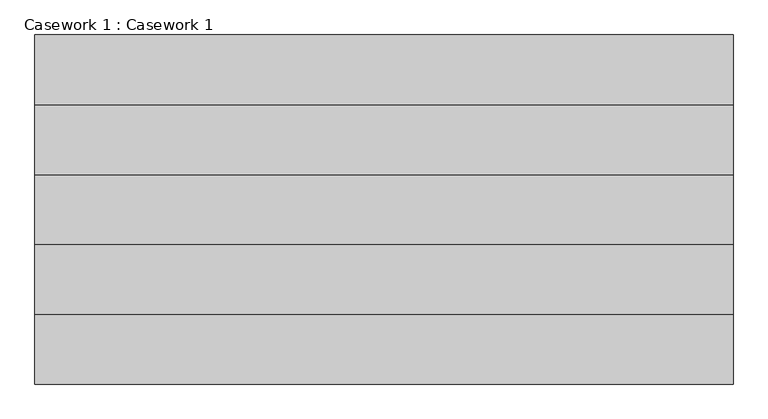
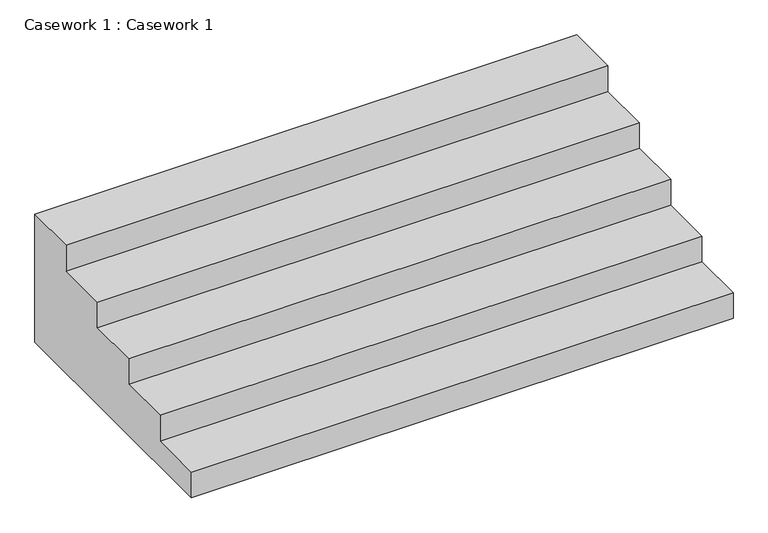
"""IFC4 building model written with IfcOpenShell, lengths in millimetres: furniture geometry, Casework 1 : Casework 1."""

from ifc_helpers import new_model, si_unit, frame, origin, place, context, project, spatial, polyline, outline, extrude, source, transform, mapped, element, save


def casework_1_casework_1_0b0e07b3(model_context):
    return source(origin(), model_context, "Body", "SweptSolid", [
        extrude(outline(polyline([(241.4737487, 2311.4), (546.2737487, 2311.4), (546.2737487, 1549.4), (-977.7262513, 1549.4), (-977.7262513, 1701.8), (-672.9262513, 1701.8), (-672.9262513, 1854.2), (-368.1262513, 1854.2), (-368.1262513, 2006.6), (-63.3262513, 2006.6), (-63.3262513, 2159.0), (241.4737487, 2159.0), (241.4737487, 2311.4)])), frame((-15445.0994093, 0.0, 0.0), z_axis=(1.0, 0.0, 0.0), x_axis=(0.0, 1.0, 0.0)), (0.0, 0.0, 1.0), 3048.0),
    ])


if __name__ == "__main__":
    model = new_model("IFC4")
    model_context = context("Model", 3, world=origin())
    ifc_project = project(units=[si_unit("LENGTHUNIT", "METRE", prefix="MILLI")], contexts=[model_context])
    site = spatial("IfcSite", under=ifc_project)
    building = spatial("IfcBuilding", under=site)
    placement = place(None, origin())
    casework_1_casework_1_shape = casework_1_casework_1_0b0e07b3(model_context)
    element("IfcFurniture", 1, ObjectType="Casework 1 : Casework 1", at=placement, inside=building, context=model_context, shape_type="MappedRepresentation", body=[
        mapped(casework_1_casework_1_shape, transform((0.0, 0.0, 0.0), x_axis=(1.0, 0.0, 0.0), y_axis=(0.0, 1.0, 0.0), z_axis=(0.0, 0.0, 1.0))),
    ])
    save(model, "model.ifc")
